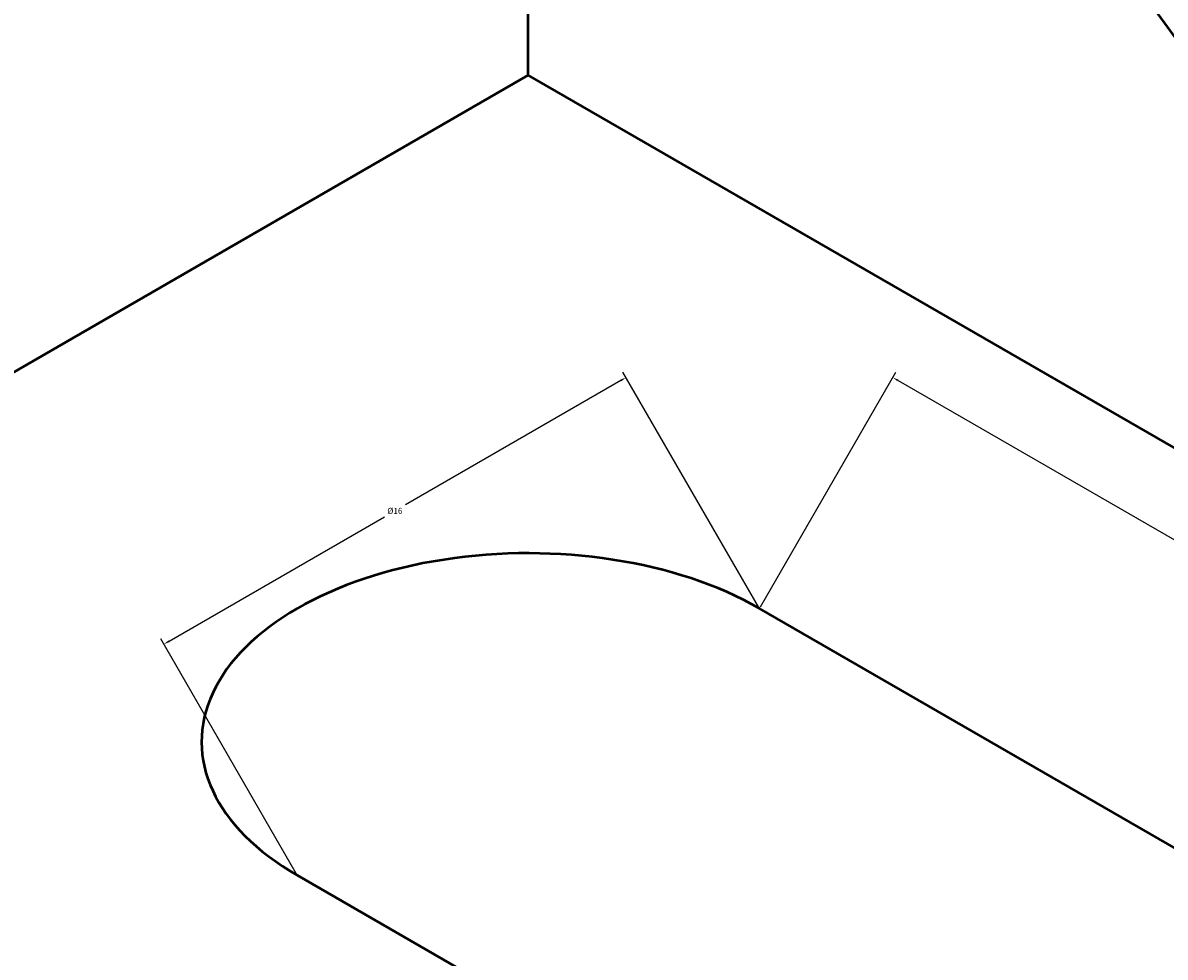
# Model space of a CAD drawing. Units: millimetres. Extents: x 2919 to 3075, y 2801 to 2951.
# Tile 12 of 14: x 3006 to 3040, y 2844 to 2872. Entities that reach past the tile are written whole.
import ezdxf

# ---------------------------------------------------------------- set-up
doc = ezdxf.new("R2010")
doc.units = ezdxf.units.MM
doc.layers.add('M-DIMS', color=2, linetype='Continuous', lineweight=18)
doc.layers.add('M-OUTL', color=7, linetype='Continuous', lineweight=50)
doc.styles.get("Standard").update_dxf_attribs({"font": 'arial.ttf'})
doc.dimstyles.get("Standard").update_dxf_attribs({"dimtxt": 0.18, "dimasz": 0.18, "dimexe": 0.18, "dimexo": 0.0625, "dimgap": 0.09, "dimtad": 0, "dimtih": 1, "dimtoh": 1, "dimdec": 4, "dimzin": 0, "dimdsep": 46, "dimtxsty": 'Standard', "dimcen": 0.09, "dimadec": 0, "dimazin": 0, "dimtfac": 1, "dimtdec": 4, "dimtofl": 0, "dimtmove": 0, "dimatfit": 3, "dimfxl": 1, "dimtolj": 1, "dimtzin": 0, "dimarcsym": 0})

# ---------------------------------------------------------------- blocks, each defined once
blk = doc.blocks.new('*D1')
at = {"layer": 'Defpoints', "color": 0, "transparency": 16777216}
for p in [(2987.323, 2944.203), (3074.337, 2944.203), (3010.912, 2808.893)]:
    blk.add_point(p, dxfattribs=at)
at = {"layer": 'M-DIMS', "color": 0, "lineweight": -2, "transparency": 16777216}
for p, q in [((2987.386, 2944.203), (3074.517, 2944.203)), ((3074.337, 2944.023), (3074.337, 2876.73)), ((3074.337, 2809.073), (3074.337, 2876.366)), ((3010.974, 2808.893), (3074.517, 2808.893))]:
    blk.add_line(p, q, dxfattribs=at)
at = {"layer": 'M-DIMS', "color": 0, "transparency": 16777216}
for points in [[(3074.307, 2944.023), (3074.367, 2944.023), (3074.337, 2944.203)], [(3074.307, 2809.073), (3074.367, 2809.073), (3074.337, 2808.893)]]:
    blk.add_solid(points, dxfattribs=at)
at = {"layer": 'M-DIMS', "color": 0, "transparency": 16777216, "insert": (3074.337, 2876.548), "char_height": 0.18, "attachment_point": 5}
blk.add_mtext('\\A1;135.3', dxfattribs=at)
blk = doc.blocks.new('*D2')
at = {"layer": 'Defpoints', "color": 0, "transparency": 16777216}
for p in [(2927.773, 2856.893), (3066.337, 2840.893), (3066.337, 2800.893)]:
    blk.add_point(p, dxfattribs=at)
at = {"layer": 'M-DIMS', "color": 0, "lineweight": -2, "transparency": 16777216}
for p, q in [((2927.773, 2856.831), (2927.773, 2800.713)), ((3066.337, 2840.831), (3066.337, 2800.713)), ((2927.953, 2800.893), (2996.6, 2800.893)), ((3066.157, 2800.893), (2997.51, 2800.893))]:
    blk.add_line(p, q, dxfattribs=at)
at = {"layer": 'M-DIMS', "color": 0, "transparency": 16777216}
for points in [[(2927.953, 2800.923), (2927.953, 2800.863), (2927.773, 2800.893)], [(3066.157, 2800.923), (3066.157, 2800.863), (3066.337, 2800.893)]]:
    blk.add_solid(points, dxfattribs=at)
at = {"layer": 'M-DIMS', "color": 0, "transparency": 16777216, "insert": (2997.055, 2800.893), "char_height": 0.18, "attachment_point": 5}
blk.add_mtext('\\A1;138.56', dxfattribs=at)
blk = doc.blocks.new('*D3')
at = {"layer": 'Defpoints', "color": 0, "transparency": 16777216}
for p in [(2927.773, 2856.893), (2923.773, 2849.965), (3010.912, 2808.893)]:
    blk.add_point(p, dxfattribs=at)
at = {"layer": 'M-DIMS', "color": 0, "lineweight": -2, "transparency": 16777216}
for p, q in [((2927.742, 2856.839), (2923.683, 2849.809)), ((2923.929, 2849.875), (2965.124, 2826.091)), ((3006.756, 2802.055), (2965.561, 2825.839)), ((3010.88, 2808.839), (3006.822, 2801.809))]:
    blk.add_line(p, q, dxfattribs=at)
at = {"layer": 'M-DIMS', "color": 0, "transparency": 16777216}
for points in [[(2923.944, 2849.901), (2923.914, 2849.849), (2923.773, 2849.965)], [(3006.771, 2802.081), (3006.741, 2802.029), (3006.912, 2801.965)]]:
    blk.add_solid(points, dxfattribs=at)
at = {"layer": 'M-DIMS', "color": 0, "transparency": 16777216, "insert": (2965.342, 2825.965), "char_height": 0.18, "attachment_point": 5}
blk.add_mtext('\\A1;96', dxfattribs=at)
blk = doc.blocks.new('*D7')
at = {"layer": 'Defpoints', "color": 0, "transparency": 16777216}
for p in [(3028.232, 2854.893), (3049.552, 2851.822), (3045.553, 2844.893)]:
    blk.add_point(p, dxfattribs=at)
at = {"layer": 'M-DIMS', "color": 0, "lineweight": -2, "transparency": 16777216}
for p, q in [((3028.263, 2854.947), (3032.321, 2861.977)), ((3032.387, 2861.731), (3040.672, 2856.948)), ((3049.397, 2851.912), (3041.112, 2856.694)), ((3045.584, 2844.947), (3049.642, 2851.977))]:
    blk.add_line(p, q, dxfattribs=at)
at = {"layer": 'M-DIMS', "color": 0, "transparency": 16777216}
for points in [[(3032.402, 2861.757), (3032.372, 2861.705), (3032.231, 2861.821)], [(3049.412, 2851.938), (3049.382, 2851.886), (3049.552, 2851.822)]]:
    blk.add_solid(points, dxfattribs=at)
at = {"layer": 'M-DIMS', "color": 0, "transparency": 16777216, "insert": (3040.892, 2856.821), "char_height": 0.18, "attachment_point": 5}
blk.add_mtext('\\A1;20', dxfattribs=at)
blk = doc.blocks.new('*D8')
at = {"layer": 'Defpoints', "color": 0, "transparency": 16777216}
for p in [(3024.232, 2861.821), (3028.232, 2854.893), (3014.376, 2846.894)]:
    blk.add_point(p, dxfattribs=at)
at = {"layer": 'M-DIMS', "color": 0, "lineweight": -2, "transparency": 16777216}
for p, q in [((3024.076, 2861.731), (3017.621, 2858.004)), ((3028.2, 2854.947), (3024.142, 2861.977)), ((3010.532, 2853.912), (3016.987, 2857.639)), ((3014.345, 2846.948), (3010.286, 2853.978))]:
    blk.add_line(p, q, dxfattribs=at)
at = {"layer": 'M-DIMS', "color": 0, "transparency": 16777216}
for points in [[(3024.061, 2861.757), (3024.091, 2861.705), (3024.232, 2861.821)], [(3010.517, 2853.938), (3010.547, 2853.886), (3010.376, 2853.822)]]:
    blk.add_solid(points, dxfattribs=at)
at = {"layer": 'M-DIMS', "color": 0, "transparency": 16777216, "insert": (3017.304, 2857.821), "char_height": 0.18, "attachment_point": 5}
blk.add_mtext('\\A1;%%c16', dxfattribs=at)

msp = doc.modelspace()

# ---------------------------------------------------------------- linework, layer by layer
at = {"layer": 'M-OUTL'}
for p, q in [((3021.3039, 2870.8932), (3021.3039, 2898.8932)), ((3055.9449, 2850.8932), (3021.3039, 2898.8932)), ((2995.3232, 2855.8932), (3021.3039, 2870.8932)), ((3055.9449, 2850.8932), (3021.3039, 2870.8932)), ((3028.2316, 2854.8929), (3028.2321, 2854.8932)), ((3045.5526, 2844.8932), (3028.2321, 2854.8932)), ((3014.3757, 2846.8932), (3014.3763, 2846.8936)), ((3031.6962, 2836.8932), (3014.3757, 2846.8932))]:
    msp.add_line(p, q, dxfattribs=at)
msp.add_ellipse((3021.3039, 2850.8932), major_axis=(-9.7972, 0), ratio=0.5773503, start_param=3.9269908, end_param=7.0685835, dxfattribs=at)

# ---------------------------------------------------------------- dimensions: what is measured, and where the dimension line sits
at = {"layer": 'M-DIMS'}
for base, p1, p2, angle, override, picture, middle in [((3074.3372, 2944.2026), (3010.9116, 2808.8932), (2987.3232, 2944.2026), 90, {"dimdec": 1, "dimlfac": 1, "dimrnd": 0, "dimzin": 0, "dimdsep": 46, "dimlunit": 2}, '*D1', (3074.3372, 2876.5479)), ((3049.5525, 2851.8216), (3028.2316, 2854.8929), (3045.5526, 2844.8932), 330.00155, {"dimdec": 0, "dimlfac": 1, "dimrnd": 0, "dimzin": 0, "dimdsep": 46, "dimlunit": 2}, '*D7', (3040.8919, 2856.8214)), ((2923.7732, 2849.965), (3010.9116, 2808.8932), (2927.7732, 2856.8932), 150, {"dimdec": 0, "dimlfac": 1, "dimrnd": 0, "dimzin": 0, "dimdsep": 46, "dimlunit": 2}, '*D3', (2965.3424, 2825.965))]:
    dim = msp.add_linear_dim(base=base, p1=p1, p2=p2, angle=angle, dimstyle='Standard', override=override, dxfattribs=at)
    dim.commit()
    dim.dimension.update_dxf_attribs({"geometry": picture, "text_midpoint": middle})
dim = msp.add_linear_dim(base=(3024.2316, 2861.8211), p1=(3014.3763, 2846.8936), p2=(3028.2316, 2854.8929), angle=30, text='%%c<>', dimstyle='Standard', override={"dimdec": 0, "dimlfac": 1, "dimrnd": 0, "dimzin": 0, "dimdsep": 46, "dimlunit": 2}, dxfattribs=at)
dim.commit()
dim.dimension.update_dxf_attribs({"geometry": '*D8', "text_midpoint": (3017.3039, 2857.8214)})
dim = msp.add_linear_dim(base=(3066.3372, 2800.8932), p1=(2927.7732, 2856.8932), p2=(3066.3372, 2840.8932), dimstyle='Standard', override={"dimdec": 2, "dimlfac": 1, "dimrnd": 0, "dimzin": 0, "dimdsep": 46, "dimlunit": 2}, dxfattribs=at)
dim.commit()
dim.dimension.update_dxf_attribs({"geometry": '*D2', "text_midpoint": (2997.0552, 2800.8932)})

doc.saveas('drawing.dxf')
